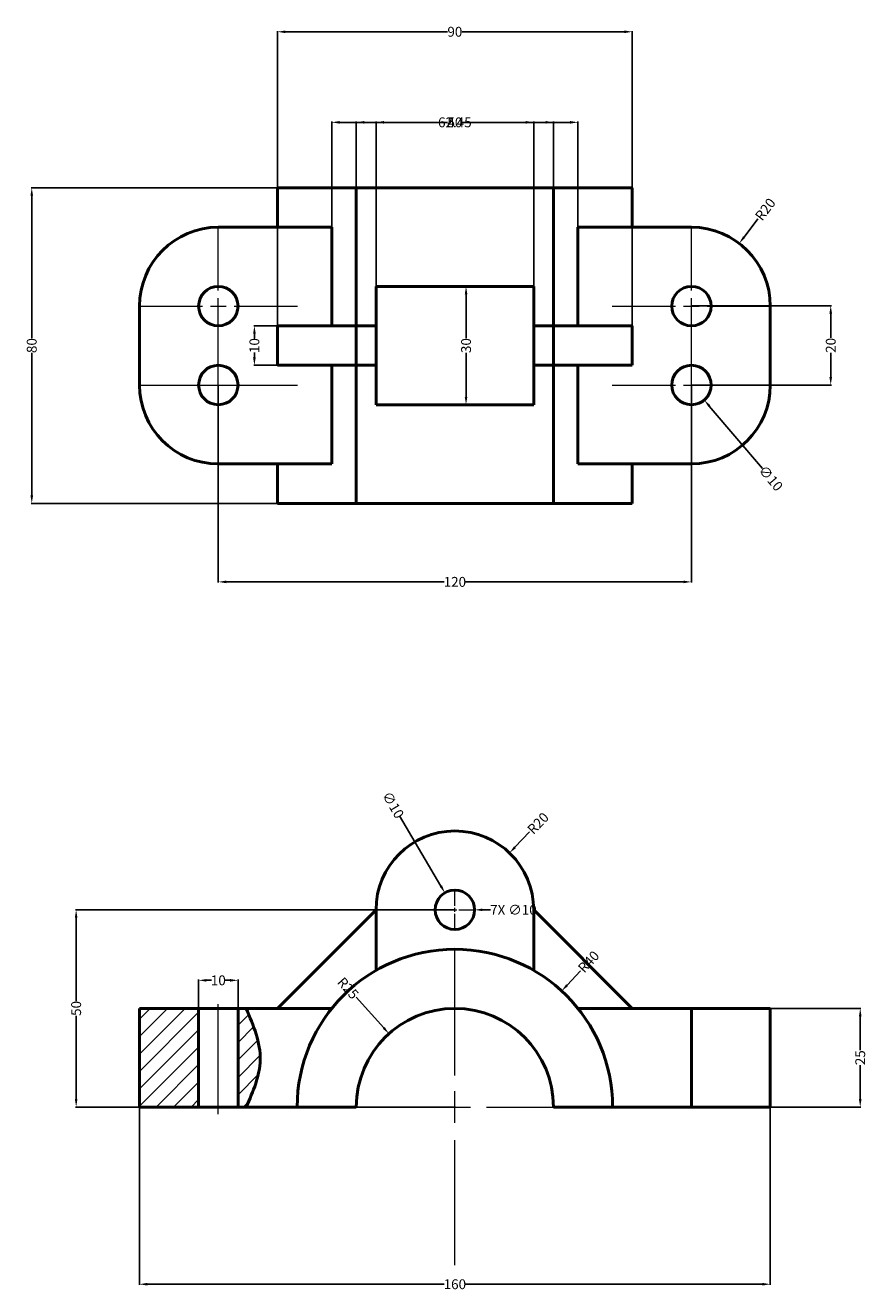
# Model space of a CAD drawing. Units: inches. Extents: x 156 to 369, y 156 to 477.
import ezdxf

# ---------------------------------------------------------------- set-up
doc = ezdxf.new("R2010")
doc.units = ezdxf.units.IN
doc.header["$MEASUREMENT"] = 0
doc.linetypes.add('CENTER', pattern=[50.8, 31.75, -6.35, 6.35, -6.35])
for name, color, linetype, lineweight in [('M-CNTR', 1, 'CENTER', 18), ('M-DIMS', 2, 'Continuous', 25), ('M-HATC', 8, 'Continuous', 18), ('M-OUTL', 7, 'Continuous', 50)]:
    doc.layers.add(name, color=color, linetype=linetype, lineweight=lineweight)
doc.styles.get("Standard").update_dxf_attribs({"font": 'arial.ttf'})
doc.dimstyles.get("Standard").update_dxf_attribs({"dimtxt": 2.5, "dimasz": 2, "dimexe": 0.18, "dimexo": 0.0625, "dimgap": 0.09, "dimtad": 0, "dimdec": 0, "dimzin": 0, "dimdsep": 46, "dimtxsty": 'Standard', "dimcen": 0.09, "dimadec": 0, "dimazin": 0, "dimtfac": 1, "dimtdec": 0, "dimtofl": 0, "dimtmove": 0, "dimatfit": 3, "dimfxl": 1, "dimtolj": 1, "dimtzin": 0, "dimarcsym": 0})

# ---------------------------------------------------------------- blocks, each defined once
blk = doc.blocks.new('*U1')
at = {"layer": 'M-CNTR', "color": 0, "transparency": 16777216}
blk.add_line((0, -14.29), (0, 13.61), dxfattribs=at)
blk = doc.blocks.new('*U2')
at = {"layer": 'M-CNTR', "color": 0, "transparency": 16777216}
for p, q in [((0, 1), (0, 5.12)), ((-5.12, 0), (-1, 0)), ((1, 0), (5.12, 0)), ((0, -5.12), (0, -1))]:
    blk.add_line(p, q, dxfattribs=at)
at = {"layer": 'M-CNTR', "color": 0, "linetype": 'Continuous', "transparency": 16777216}
for p, q in [((-0.5, 0), (0.5, 0)), ((0, -0.5), (0, 0.5))]:
    blk.add_line(p, q, dxfattribs=at)
blk = doc.blocks.new('*U3')
at = {"layer": 'M-CNTR', "color": 0, "transparency": 16777216}
for p, q in [((0, 4), (0, 20.12)), ((-20.12, 0), (-4, 0)), ((4, 0), (20.12, 0)), ((0, -20.12), (0, -4))]:
    blk.add_line(p, q, dxfattribs=at)
at = {"layer": 'M-CNTR', "color": 0, "linetype": 'Continuous', "transparency": 16777216}
for p, q in [((-2, 0), (2, 0)), ((0, -2), (0, 2))]:
    blk.add_line(p, q, dxfattribs=at)
blk = doc.blocks.new('*U4')
at = {"layer": 'M-CNTR', "color": 0, "transparency": 16777216}
for p, q in [((0, 4), (0, 20.12)), ((-20.12, 0), (-4, 0)), ((4, 0), (20.12, 0)), ((0, -20.12), (0, -4))]:
    blk.add_line(p, q, dxfattribs=at)
at = {"layer": 'M-CNTR', "color": 0, "linetype": 'Continuous', "transparency": 16777216}
for p, q in [((-2, 0), (2, 0)), ((0, -2), (0, 2))]:
    blk.add_line(p, q, dxfattribs=at)
blk = doc.blocks.new('*U5')
at = {"layer": 'M-CNTR', "color": 0, "transparency": 16777216}
for p, q in [((0, 4), (0, 20.12)), ((-20.12, 0), (-4, 0)), ((4, 0), (20.12, 0)), ((0, -20.12), (0, -4))]:
    blk.add_line(p, q, dxfattribs=at)
at = {"layer": 'M-CNTR', "color": 0, "linetype": 'Continuous', "transparency": 16777216}
for p, q in [((-2, 0), (2, 0)), ((0, -2), (0, 2))]:
    blk.add_line(p, q, dxfattribs=at)
blk = doc.blocks.new('*U6')
at = {"layer": 'M-CNTR', "color": 0, "transparency": 16777216}
for p, q in [((0, 4), (0, 20.12)), ((-20.12, 0), (-4, 0)), ((4, 0), (20.12, 0)), ((0, -20.12), (0, -4))]:
    blk.add_line(p, q, dxfattribs=at)
at = {"layer": 'M-CNTR', "color": 0, "linetype": 'Continuous', "transparency": 16777216}
for p, q in [((-2, 0), (2, 0)), ((0, -2), (0, 2))]:
    blk.add_line(p, q, dxfattribs=at)
blk = doc.blocks.new('*U7')
at = {"layer": 'M-CNTR', "color": 0, "transparency": 16777216}
for p, q in [((0, 1), (0, 5.12)), ((-5.12, 0), (-1, 0)), ((1, 0), (5.12, 0)), ((0, -5.12), (0, -1))]:
    blk.add_line(p, q, dxfattribs=at)
at = {"layer": 'M-CNTR', "color": 0, "linetype": 'Continuous', "transparency": 16777216}
for p, q in [((-0.5, 0), (0.5, 0)), ((0, -0.5), (0, 0.5))]:
    blk.add_line(p, q, dxfattribs=at)
blk = doc.blocks.new('*U8')
at = {"layer": 'M-CNTR', "color": 0, "transparency": 16777216}
for p, q in [((0, 8), (0, 40.12)), ((-40.12, 0), (-8, 0)), ((8, 0), (40.12, 0)), ((0, -40.12), (0, -8))]:
    blk.add_line(p, q, dxfattribs=at)
at = {"layer": 'M-CNTR', "color": 0, "linetype": 'Continuous', "transparency": 16777216}
for p, q in [((0, -4), (0, 4)), ((-4, 0), (4, 0))]:
    blk.add_line(p, q, dxfattribs=at)
blk = doc.blocks.new('*D9')
at = {"layer": 'Defpoints', "color": 0, "transparency": 16777216}
for p in [(184.76, 202.26), (344.76, 202.26), (344.76, 157.33)]:
    blk.add_point(p, dxfattribs=at)
at = {"layer": 'M-DIMS', "color": 0, "lineweight": -2, "transparency": 16777216}
for p, q in [((184.76, 202.19), (184.76, 157.15)), ((344.76, 202.19), (344.76, 157.15)), ((186.76, 157.33), (262.03, 157.33)), ((342.76, 157.33), (267.49, 157.33))]:
    blk.add_line(p, q, dxfattribs=at)
at = {"layer": 'M-DIMS', "color": 0, "transparency": 16777216}
for points in [[(186.76, 157.67), (186.76, 157), (184.76, 157.33)], [(342.76, 157.67), (342.76, 157), (344.76, 157.33)]]:
    blk.add_solid(points, dxfattribs=at)
at = {"layer": 'M-DIMS', "color": 0, "transparency": 16777216, "insert": (264.76, 157.33), "char_height": 2.5, "attachment_point": 5}
blk.add_mtext('\\A1;160', dxfattribs=at)
blk = doc.blocks.new('*D10')
at = {"layer": 'Defpoints', "color": 0, "transparency": 16777216}
for p in [(344.76, 227.26), (367.58, 227.26), (344.76, 202.26)]:
    blk.add_point(p, dxfattribs=at)
at = {"layer": 'M-DIMS', "color": 0, "lineweight": -2, "transparency": 16777216}
for p, q in [((344.83, 227.26), (367.76, 227.26)), ((367.58, 225.26), (367.58, 216.67)), ((367.58, 204.26), (367.58, 212.84)), ((344.83, 202.26), (367.76, 202.26))]:
    blk.add_line(p, q, dxfattribs=at)
at = {"layer": 'M-DIMS', "color": 0, "transparency": 16777216}
for points in [[(367.25, 225.26), (367.91, 225.26), (367.58, 227.26)], [(367.25, 204.26), (367.91, 204.26), (367.58, 202.26)]]:
    blk.add_solid(points, dxfattribs=at)
at = {"layer": 'M-DIMS', "color": 0, "transparency": 16777216, "insert": (367.58, 214.76), "char_height": 2.5, "attachment_point": 5, "rotation": 90}
blk.add_mtext('\\A1;25', dxfattribs=at)
blk = doc.blocks.new('*D11')
at = {"layer": 'Defpoints', "color": 0, "transparency": 16777216}
for p in [(264.76, 252.26), (168.7, 202.26), (264.76, 202.26)]:
    blk.add_point(p, dxfattribs=at)
at = {"layer": 'M-DIMS', "color": 0, "lineweight": -2, "transparency": 16777216}
for p, q in [((264.7, 252.26), (168.52, 252.26)), ((168.7, 250.26), (168.7, 229.13)), ((168.7, 204.26), (168.7, 225.38)), ((264.7, 202.26), (168.52, 202.26))]:
    blk.add_line(p, q, dxfattribs=at)
at = {"layer": 'M-DIMS', "color": 0, "transparency": 16777216}
for points in [[(168.37, 250.26), (169.03, 250.26), (168.7, 252.26)], [(168.37, 204.26), (169.03, 204.26), (168.7, 202.26)]]:
    blk.add_solid(points, dxfattribs=at)
at = {"layer": 'M-DIMS', "color": 0, "transparency": 16777216, "insert": (168.7, 227.26), "char_height": 2.5, "attachment_point": 5, "rotation": 90}
blk.add_mtext('\\A1;50', dxfattribs=at)
blk = doc.blocks.new('*D12')
at = {"layer": 'Defpoints', "color": 0, "transparency": 16777216}
for p in [(209.76, 234.38), (199.76, 227.26), (209.76, 227.26)]:
    blk.add_point(p, dxfattribs=at)
at = {"layer": 'M-DIMS', "color": 0, "lineweight": -2, "transparency": 16777216}
for p, q in [((199.76, 227.32), (199.76, 234.56)), ((201.76, 234.38), (203, 234.38)), ((207.76, 234.38), (206.52, 234.38)), ((209.76, 227.32), (209.76, 234.56))]:
    blk.add_line(p, q, dxfattribs=at)
at = {"layer": 'M-DIMS', "color": 0, "transparency": 16777216}
for points in [[(201.76, 234.71), (201.76, 234.04), (199.76, 234.38)], [(207.76, 234.71), (207.76, 234.04), (209.76, 234.38)]]:
    blk.add_solid(points, dxfattribs=at)
at = {"layer": 'M-DIMS', "color": 0, "transparency": 16777216, "insert": (204.76, 234.38), "char_height": 2.5, "attachment_point": 5}
blk.add_mtext('\\A1;10', dxfattribs=at)
blk = doc.blocks.new('*D13')
at = {"layer": 'Defpoints', "color": 0, "transparency": 16777216}
for p in [(278.62, 266.68), (264.76, 252.26)]:
    blk.add_point(p, dxfattribs=at)
at = {"layer": 'M-DIMS', "color": 0, "lineweight": -2, "transparency": 16777216}
for p, q in [((283.73, 271.99), (280.01, 268.12)), ((264.67, 252.26), (264.85, 252.26)), ((264.76, 252.17), (264.76, 252.35))]:
    blk.add_line(p, q, dxfattribs=at)
at = {"layer": 'M-DIMS', "color": 0, "transparency": 16777216}
blk.add_solid([(279.77, 268.35), (280.25, 267.89), (278.62, 266.68)], dxfattribs=at)
at = {"layer": 'M-DIMS', "color": 0, "transparency": 16777216, "insert": (285.86, 274.2), "char_height": 2.5, "attachment_point": 5, "rotation": 46.136}
blk.add_mtext('\\A1;R20', dxfattribs=at)
blk = doc.blocks.new('*D14')
at = {"layer": 'Defpoints', "color": 0, "transparency": 16777216}
for p in [(291.86, 231.68), (264.76, 202.26)]:
    blk.add_point(p, dxfattribs=at)
at = {"layer": 'M-DIMS', "color": 0, "lineweight": -2, "transparency": 16777216}
for p, q in [((296.61, 236.83), (293.22, 233.15)), ((264.67, 202.26), (264.85, 202.26)), ((264.76, 202.17), (264.76, 202.35))]:
    blk.add_line(p, q, dxfattribs=at)
at = {"layer": 'M-DIMS', "color": 0, "transparency": 16777216}
blk.add_solid([(292.97, 233.37), (293.46, 232.92), (291.86, 231.68)], dxfattribs=at)
at = {"layer": 'M-DIMS', "color": 0, "transparency": 16777216, "insert": (298.69, 239.09), "char_height": 2.5, "attachment_point": 5, "rotation": 47.3487}
blk.add_mtext('\\A1;R40', dxfattribs=at)
blk = doc.blocks.new('*D15')
at = {"layer": 'Defpoints', "color": 0, "transparency": 16777216}
for p in [(248.05, 220.84), (264.76, 202.26)]:
    blk.add_point(p, dxfattribs=at)
at = {"layer": 'M-DIMS', "color": 0, "lineweight": -2, "transparency": 16777216}
for p, q in [((239.72, 230.1), (246.71, 222.33)), ((264.67, 202.26), (264.85, 202.26)), ((264.76, 202.17), (264.76, 202.35))]:
    blk.add_line(p, q, dxfattribs=at)
at = {"layer": 'M-DIMS', "color": 0, "transparency": 16777216}
blk.add_solid([(246.96, 222.55), (246.46, 222.11), (248.05, 220.84)], dxfattribs=at)
at = {"layer": 'M-DIMS', "color": 0, "transparency": 16777216, "insert": (237.66, 232.4), "char_height": 2.5, "attachment_point": 5, "rotation": 311.9649}
blk.add_mtext('\\A1;R25', dxfattribs=at)
blk = doc.blocks.new('*D16')
at = {"layer": 'Defpoints', "color": 0, "transparency": 16777216}
for p in [(262.23, 256.56), (267.3, 247.95)]:
    blk.add_point(p, dxfattribs=at)
at = {"layer": 'M-DIMS', "color": 0, "lineweight": -2, "transparency": 16777216}
for p, q in [((250.75, 276.06), (261.21, 258.29)), ((264.67, 252.26), (264.85, 252.26)), ((264.76, 252.17), (264.76, 252.35))]:
    blk.add_line(p, q, dxfattribs=at)
at = {"layer": 'M-DIMS', "color": 0, "transparency": 16777216}
blk.add_solid([(261.5, 258.46), (260.92, 258.12), (262.23, 256.56)], dxfattribs=at)
at = {"layer": 'M-DIMS', "color": 0, "transparency": 16777216, "insert": (249.11, 278.85), "char_height": 2.5, "attachment_point": 5, "rotation": 300.4828}
blk.add_mtext('\\A1;∅10', dxfattribs=at)
blk = doc.blocks.new('*D17')
at = {"layer": 'Defpoints', "color": 0, "transparency": 16777216}
for p in [(204.76, 385.31), (324.76, 385.31), (324.76, 335.4)]:
    blk.add_point(p, dxfattribs=at)
at = {"layer": 'M-DIMS', "color": 0, "lineweight": -2, "transparency": 16777216}
for p, q in [((204.76, 385.25), (204.76, 335.22)), ((324.76, 385.25), (324.76, 335.22)), ((206.76, 335.4), (262.03, 335.4)), ((322.76, 335.4), (267.49, 335.4))]:
    blk.add_line(p, q, dxfattribs=at)
at = {"layer": 'M-DIMS', "color": 0, "transparency": 16777216}
for points in [[(206.76, 335.73), (206.76, 335.06), (204.76, 335.4)], [(322.76, 335.73), (322.76, 335.06), (324.76, 335.4)]]:
    blk.add_solid(points, dxfattribs=at)
at = {"layer": 'M-DIMS', "color": 0, "transparency": 16777216, "insert": (264.76, 335.4), "char_height": 2.5, "attachment_point": 5}
blk.add_mtext('\\A1;120', dxfattribs=at)
blk = doc.blocks.new('*D18')
at = {"layer": 'Defpoints', "color": 0, "transparency": 16777216}
for p in [(324.76, 405.43), (324.76, 385.31), (360.1, 385.31)]:
    blk.add_point(p, dxfattribs=at)
at = {"layer": 'M-DIMS', "color": 0, "lineweight": -2, "transparency": 16777216}
for p, q in [((324.83, 405.43), (360.28, 405.43)), ((360.1, 403.43), (360.1, 397.27)), ((360.1, 387.31), (360.1, 393.48)), ((324.83, 385.31), (360.28, 385.31))]:
    blk.add_line(p, q, dxfattribs=at)
at = {"layer": 'M-DIMS', "color": 0, "transparency": 16777216}
for points in [[(359.76, 403.43), (360.43, 403.43), (360.1, 405.43)], [(359.76, 387.31), (360.43, 387.31), (360.1, 385.31)]]:
    blk.add_solid(points, dxfattribs=at)
at = {"layer": 'M-DIMS', "color": 0, "transparency": 16777216, "insert": (360.1, 395.37), "char_height": 2.5, "attachment_point": 5, "rotation": 90}
blk.add_mtext('\\A1;20', dxfattribs=at)
blk = doc.blocks.new('*D19')
at = {"layer": 'Defpoints', "color": 0, "transparency": 16777216}
for p in [(309.76, 474.87), (219.76, 395.31), (309.76, 395.31)]:
    blk.add_point(p, dxfattribs=at)
at = {"layer": 'M-DIMS', "color": 0, "lineweight": -2, "transparency": 16777216}
for p, q in [((219.76, 395.38), (219.76, 475.05)), ((221.76, 474.87), (262.89, 474.87)), ((307.76, 474.87), (266.64, 474.87)), ((309.76, 395.38), (309.76, 475.05))]:
    blk.add_line(p, q, dxfattribs=at)
at = {"layer": 'M-DIMS', "color": 0, "transparency": 16777216}
for points in [[(221.76, 475.2), (221.76, 474.54), (219.76, 474.87)], [(307.76, 475.2), (307.76, 474.54), (309.76, 474.87)]]:
    blk.add_solid(points, dxfattribs=at)
at = {"layer": 'M-DIMS', "color": 0, "transparency": 16777216, "insert": (264.76, 474.87), "char_height": 2.5, "attachment_point": 5}
blk.add_mtext('\\A1;90', dxfattribs=at)
blk = doc.blocks.new('*D20')
at = {"layer": 'Defpoints', "color": 0, "transparency": 16777216}
for p in [(219.76, 435.31), (157.44, 355.31), (219.76, 355.31)]:
    blk.add_point(p, dxfattribs=at)
at = {"layer": 'M-DIMS', "color": 0, "lineweight": -2, "transparency": 16777216}
for p, q in [((219.7, 435.31), (157.26, 435.31)), ((157.44, 433.31), (157.44, 397.19)), ((157.44, 357.31), (157.44, 393.44)), ((219.7, 355.31), (157.26, 355.31))]:
    blk.add_line(p, q, dxfattribs=at)
at = {"layer": 'M-DIMS', "color": 0, "transparency": 16777216}
for points in [[(157.11, 433.31), (157.78, 433.31), (157.44, 435.31)], [(157.11, 357.31), (157.78, 357.31), (157.44, 355.31)]]:
    blk.add_solid(points, dxfattribs=at)
at = {"layer": 'M-DIMS', "color": 0, "transparency": 16777216, "insert": (157.44, 395.31), "char_height": 2.5, "attachment_point": 5, "rotation": 90}
blk.add_mtext('\\A1;80', dxfattribs=at)
blk = doc.blocks.new('*D21')
at = {"layer": 'Defpoints', "color": 0, "transparency": 16777216}
for p in [(284.76, 410.31), (267.6, 380.31), (284.76, 380.31)]:
    blk.add_point(p, dxfattribs=at)
at = {"layer": 'M-DIMS', "color": 0, "lineweight": -2, "transparency": 16777216}
for p, q in [((284.7, 410.31), (267.42, 410.31)), ((267.6, 408.31), (267.6, 397.19)), ((267.6, 382.31), (267.6, 393.44)), ((284.7, 380.31), (267.42, 380.31))]:
    blk.add_line(p, q, dxfattribs=at)
at = {"layer": 'M-DIMS', "color": 0, "transparency": 16777216}
for points in [[(267.27, 408.31), (267.93, 408.31), (267.6, 410.31)], [(267.27, 382.31), (267.93, 382.31), (267.6, 380.31)]]:
    blk.add_solid(points, dxfattribs=at)
at = {"layer": 'M-DIMS', "color": 0, "transparency": 16777216, "insert": (267.6, 395.31), "char_height": 2.5, "attachment_point": 5, "rotation": 90}
blk.add_mtext('\\A1;30', dxfattribs=at)
blk = doc.blocks.new('*D22')
at = {"layer": 'Defpoints', "color": 0, "transparency": 16777216}
for p in [(219.76, 400.31), (213.91, 390.31), (219.76, 390.31)]:
    blk.add_point(p, dxfattribs=at)
at = {"layer": 'M-DIMS', "color": 0, "lineweight": -2, "transparency": 16777216}
for p, q in [((219.7, 400.31), (213.73, 400.31)), ((213.91, 398.31), (213.91, 397.07)), ((213.91, 392.31), (213.91, 393.55)), ((219.7, 390.31), (213.73, 390.31))]:
    blk.add_line(p, q, dxfattribs=at)
at = {"layer": 'M-DIMS', "color": 0, "transparency": 16777216}
for points in [[(213.58, 398.31), (214.25, 398.31), (213.91, 400.31)], [(213.58, 392.31), (214.25, 392.31), (213.91, 390.31)]]:
    blk.add_solid(points, dxfattribs=at)
at = {"layer": 'M-DIMS', "color": 0, "transparency": 16777216, "insert": (213.91, 395.31), "char_height": 2.5, "attachment_point": 5, "rotation": 90}
blk.add_mtext('\\A1;10', dxfattribs=at)
blk = doc.blocks.new('*D23')
at = {"layer": 'Defpoints', "color": 0, "transparency": 16777216}
for p in [(336.9, 421.21), (324.76, 405.31)]:
    blk.add_point(p, dxfattribs=at)
at = {"layer": 'M-DIMS', "color": 0, "lineweight": -2, "transparency": 16777216}
for p, q in [((341.63, 427.42), (338.11, 422.8)), ((324.67, 405.31), (324.85, 405.31)), ((324.76, 405.22), (324.76, 405.4))]:
    blk.add_line(p, q, dxfattribs=at)
at = {"layer": 'M-DIMS', "color": 0, "transparency": 16777216}
blk.add_solid([(337.84, 423.01), (338.37, 422.6), (336.9, 421.21)], dxfattribs=at)
at = {"layer": 'M-DIMS', "color": 0, "transparency": 16777216, "insert": (343.5, 429.87), "char_height": 2.5, "attachment_point": 5, "rotation": 52.6551}
blk.add_mtext('\\A1;R20', dxfattribs=at)
blk = doc.blocks.new('*D24')
at = {"layer": 'Defpoints', "color": 0, "transparency": 16777216}
for p in [(321.52, 389.12), (328.01, 381.51)]:
    blk.add_point(p, dxfattribs=at)
at = {"layer": 'M-DIMS', "color": 0, "lineweight": -2, "transparency": 16777216}
for p, q in [((324.67, 385.31), (324.85, 385.31)), ((324.76, 385.22), (324.76, 385.4)), ((342.8, 364.14), (329.3, 379.99))]:
    blk.add_line(p, q, dxfattribs=at)
at = {"layer": 'M-DIMS', "color": 0, "transparency": 16777216}
blk.add_solid([(329.56, 380.2), (329.05, 379.77), (328.01, 381.51)], dxfattribs=at)
at = {"layer": 'M-DIMS', "color": 0, "transparency": 16777216, "insert": (344.9, 361.68), "char_height": 2.5, "attachment_point": 5, "rotation": 310.4308}
blk.add_mtext('\\A1;∅10', dxfattribs=at)
blk = doc.blocks.new('*D25')
at = {"layer": 'Defpoints', "color": 0, "transparency": 16777216}
for p in [(284.76, 451.91), (244.76, 410.31), (284.76, 410.31)]:
    blk.add_point(p, dxfattribs=at)
at = {"layer": 'M-DIMS', "color": 0, "lineweight": -2, "transparency": 16777216}
for p, q in [((244.76, 410.38), (244.76, 452.09)), ((246.76, 451.91), (262.84, 451.91)), ((282.76, 451.91), (266.69, 451.91)), ((284.76, 410.38), (284.76, 452.09))]:
    blk.add_line(p, q, dxfattribs=at)
at = {"layer": 'M-DIMS', "color": 0, "transparency": 16777216}
for points in [[(246.76, 452.25), (246.76, 451.58), (244.76, 451.91)], [(282.76, 452.25), (282.76, 451.58), (284.76, 451.91)]]:
    blk.add_solid(points, dxfattribs=at)
at = {"layer": 'M-DIMS', "color": 0, "transparency": 16777216, "insert": (264.76, 451.91), "char_height": 2.5, "attachment_point": 5}
blk.add_mtext('\\A1;40', dxfattribs=at)
blk = doc.blocks.new('*D26')
at = {"layer": 'Defpoints', "color": 0, "transparency": 16777216}
for p in [(289.76, 451.91), (239.76, 435.31), (289.76, 435.31)]:
    blk.add_point(p, dxfattribs=at)
at = {"layer": 'M-DIMS', "color": 0, "lineweight": -2, "transparency": 16777216}
for p, q in [((239.76, 435.38), (239.76, 452.09)), ((241.76, 451.91), (262.89, 451.91)), ((287.76, 451.91), (266.64, 451.91)), ((289.76, 435.38), (289.76, 452.09))]:
    blk.add_line(p, q, dxfattribs=at)
at = {"layer": 'M-DIMS', "color": 0, "transparency": 16777216}
for points in [[(241.76, 452.25), (241.76, 451.58), (239.76, 451.91)], [(287.76, 452.25), (287.76, 451.58), (289.76, 451.91)]]:
    blk.add_solid(points, dxfattribs=at)
at = {"layer": 'M-DIMS', "color": 0, "transparency": 16777216, "insert": (264.76, 451.91), "char_height": 2.5, "attachment_point": 5}
blk.add_mtext('\\A1;50', dxfattribs=at)
blk = doc.blocks.new('*D27')
at = {"layer": 'Defpoints', "color": 0, "transparency": 16777216}
for p in [(295.99, 451.91), (233.54, 425.31), (295.99, 425.31)]:
    blk.add_point(p, dxfattribs=at)
at = {"layer": 'M-DIMS', "color": 0, "lineweight": -2, "transparency": 16777216}
for p, q in [((233.54, 425.38), (233.54, 452.09)), ((235.54, 451.91), (260.44, 451.91)), ((293.99, 451.91), (269.09, 451.91)), ((295.99, 425.38), (295.99, 452.09))]:
    blk.add_line(p, q, dxfattribs=at)
at = {"layer": 'M-DIMS', "color": 0, "transparency": 16777216}
for points in [[(235.54, 452.25), (235.54, 451.58), (233.54, 451.91)], [(293.99, 452.25), (293.99, 451.58), (295.99, 451.91)]]:
    blk.add_solid(points, dxfattribs=at)
at = {"layer": 'M-DIMS', "color": 0, "transparency": 16777216, "insert": (264.76, 451.91), "char_height": 2.5, "attachment_point": 5}
blk.add_mtext('\\A1;62.45', dxfattribs=at)
blk = doc.blocks.new('*D28')
at = {"layer": 'Defpoints', "color": 0, "transparency": 16777216}
for p in [(259.76, 252.26), (269.76, 252.25)]:
    blk.add_point(p, dxfattribs=at)
at = {"layer": 'M-DIMS', "color": 0, "lineweight": -2, "transparency": 16777216}
for p, q in [((264.67, 252.26), (264.85, 252.26)), ((264.76, 252.17), (264.76, 252.35)), ((273.76, 252.25), (271.76, 252.25))]:
    blk.add_line(p, q, dxfattribs=at)
at = {"layer": 'M-DIMS', "color": 0, "transparency": 16777216}
blk.add_solid([(271.76, 252.59), (271.76, 251.92), (269.76, 252.25)], dxfattribs=at)
at = {"layer": 'M-DIMS', "color": 0, "transparency": 16777216, "insert": (279.61, 252.25), "char_height": 2.5, "attachment_point": 5, "rotation": 359.9947}
blk.add_mtext('\\A1;7X ∅10', dxfattribs=at)

msp = doc.modelspace()

# ---------------------------------------------------------------- hatches: boundary and pattern name
at = {"layer": 'M-HATC'}
h = msp.add_hatch(dxfattribs=at)
h.set_pattern_fill('ANSI31', color=256, scale=25)
edge = h.paths.add_edge_path()
edge.add_spline(control_points=[(211.829, 202.255), (213.575, 206.24), (217.21, 214.532), (213.669, 222.905), (211.829, 227.255)], knot_values=[0, 0, 0, 0, 12.4957208, 26.0084045, 26.0084045, 26.0084045, 26.0084045], degree=3, periodic=0)
edge.add_line((211.829, 227.255), (209.763, 227.255))
edge.add_line((209.763, 227.255), (209.763, 202.255))
edge.add_line((209.763, 202.255), (211.829, 202.255))
h.paths.add_polyline_path([(199.763, 227.255), (194.763, 227.255), (184.763, 227.255), (184.763, 202.255), (199.763, 202.255)])

# ---------------------------------------------------------------- linework, layer by layer
at = {"layer": 'M-OUTL'}
for p, q in [((219.763, 435.314), (309.763, 435.314)), ((219.763, 425.314), (219.763, 435.314)), ((219.763, 425.314), (219.763, 435.314)), ((239.763, 435.314), (239.763, 355.314)), ((289.763, 435.314), (289.763, 355.314)), ((309.763, 425.314), (309.763, 435.314)), ((309.763, 425.314), (309.763, 435.314)), ((233.538, 425.314), (204.763, 425.314)), ((233.538, 425.314), (233.538, 400.314)), ((233.538, 400.314), (233.538, 425.314)), ((233.538, 400.314), (233.538, 425.314)), ((295.988, 400.314), (295.988, 425.314)), ((295.988, 425.314), (324.763, 425.314)), ((284.763, 410.314), (244.763, 410.314)), ((244.763, 380.314), (244.763, 410.314)), ((284.763, 380.314), (284.763, 410.314)), ((184.763, 385.314), (184.763, 405.314)), ((344.763, 385.314), (344.763, 405.314)), ((244.763, 400.314), (219.763, 400.314)), ((219.763, 390.314), (219.763, 400.314)), ((219.763, 390.314), (219.763, 400.314)), ((309.763, 400.314), (284.763, 400.314)), ((284.763, 400.314), (309.763, 400.314)), ((309.763, 390.314), (309.763, 400.314)), ((219.763, 395.314), (219.763, 390.314)), ((309.763, 395.314), (309.763, 390.314)), ((244.763, 390.314), (219.763, 390.314)), ((233.538, 365.314), (233.538, 390.314)), ((233.538, 365.314), (233.538, 390.314)), ((309.763, 390.314), (284.763, 390.314)), ((284.763, 390.314), (309.763, 390.314)), ((295.988, 365.314), (295.988, 390.314)), ((244.763, 380.314), (284.763, 380.314)), ((219.763, 365.314), (204.763, 365.314)), ((219.763, 355.314), (219.763, 365.314)), ((219.763, 355.314), (219.763, 365.314)), ((219.763, 365.314), (233.538, 365.314)), ((309.763, 365.314), (295.988, 365.314)), ((309.763, 355.314), (309.763, 365.314)), ((309.763, 355.314), (309.763, 365.314)), ((309.763, 365.314), (324.763, 365.314)), ((264.763, 355.314), (219.763, 355.314)), ((219.763, 355.314), (269.141, 355.314)), ((309.763, 355.314), (260.385, 355.314)), ((309.763, 355.314), (264.763, 355.314)), ((264.763, 355.314), (309.763, 355.314)), ((244.763, 252.255), (219.763, 227.255)), ((244.763, 252.255), (244.763, 236.896)), ((244.763, 252.255), (244.763, 236.896)), ((269.763, 252.255), (269.762, 252.316)), ((284.763, 252.255), (309.763, 227.255)), ((284.763, 252.255), (284.763, 236.896)), ((284.763, 252.255), (284.763, 236.896)), ((184.763, 202.255), (184.763, 227.255)), ((184.763, 227.255), (194.763, 227.255)), ((199.763, 202.255), (199.763, 227.255)), ((209.763, 202.255), (209.763, 227.255)), ((324.763, 202.255), (324.763, 227.255)), ((344.763, 227.255), (334.763, 227.255)), ((344.763, 202.255), (344.763, 227.255)), ((204.763, 202.255), (184.763, 202.255)), ((211.829, 202.255), (204.763, 202.255))]:
    msp.add_line(p, q, dxfattribs=at)
for points in [[(194.763, 227.255), (233.538, 227.255)], [(295.988, 227.255), (334.763, 227.255)], [(239.763, 202.255), (194.763, 202.255)], [(324.763, 202.255), (289.763, 202.255)], [(344.763, 202.255), (324.763, 202.255)]]:
    msp.add_lwpolyline(points, dxfattribs=at)
for centre in [(204.763, 405.314), (324.763, 405.314), (324.763, 405.314), (204.763, 385.314), (324.763, 385.314), (324.763, 385.314), (264.763, 252.255)]:
    msp.add_circle(centre, 5, dxfattribs=at)
for centre, radius, start, end in [((204.763, 405.314), 20, 90, 180), ((324.763, 405.314), 20, 360, 90), ((204.763, 385.314), 20, 180, 270), ((324.763, 385.314), 20, 270, 360), ((264.763, 252.255), 20, 0, 180), ((264.763, 202.255), 40, 0, 180), ((264.763, 202.255), 25, 0, 180)]:
    msp.add_arc(centre, radius, start, end, dxfattribs=at)
msp.add_open_spline([(211.829, 227.255), (213.669, 222.905), (217.21, 214.532), (213.575, 206.24), (211.829, 202.255)], degree=3, knots=[0, 0, 0, 0, 13.5126838, 26.0084045, 26.0084045, 26.0084045, 26.0084045], dxfattribs=at)

# ---------------------------------------------------------------- block references
at = {"layer": 'M-CNTR'}
for name, p in [('*U4', (204.763, 405.314)), ('*U5', (324.763, 405.314)), ('*U3', (204.763, 385.314)), ('*U6', (324.763, 385.314)), ('*U2', (204.763, 385.314)), ('*U7', (264.763, 252.255)), ('*U8', (264.763, 202.255)), ('*U1', (204.763, 214.755))]:
    msp.add_blockref(name, p, dxfattribs=at)

# ---------------------------------------------------------------- dimensions: what is measured, and where the dimension line sits
at = {"layer": 'M-DIMS'}
for base, p1, p2, override, picture, middle in [((309.763, 474.871), (219.763, 395.314), (309.763, 395.314), {"dimclrd": 0, "dimclre": 0, "dimclrt": 0}, '*D19', (264.763, 474.871)), ((295.988, 451.914), (233.538, 425.314), (295.988, 425.314), {"dimdec": 2, "dimlfac": 1, "dimrnd": 0, "dimzin": 0, "dimdsep": 46, "dimlunit": 2}, '*D27', (264.763, 451.914)), ((289.763, 451.914), (239.763, 435.314), (289.763, 435.314), {"dimdec": 0, "dimlfac": 1, "dimrnd": 0, "dimzin": 0, "dimdsep": 46, "dimlunit": 2}, '*D26', (264.763, 451.914)), ((284.763, 451.914), (244.763, 410.314), (284.763, 410.314), {"dimdec": 0, "dimlfac": 1, "dimrnd": 0, "dimzin": 0, "dimdsep": 46, "dimlunit": 2}, '*D25', (264.763, 451.914)), ((324.763, 335.396), (204.763, 385.314), (324.763, 385.314), {"dimclrd": 0, "dimclre": 0, "dimclrt": 0}, '*D17', (264.763, 335.396)), ((209.763, 234.376), (199.763, 227.255), (209.763, 227.255), {"dimclrd": 0, "dimclre": 0, "dimclrt": 0}, '*D12', (204.763, 234.376)), ((344.763, 157.333), (184.763, 202.255), (344.763, 202.255), {"dimclrd": 0, "dimclre": 0, "dimclrt": 0}, '*D9', (264.763, 157.333))]:
    dim = msp.add_linear_dim(base=base, p1=p1, p2=p2, dimstyle='Standard', override=override, dxfattribs=at)
    dim.commit()
    dim.dimension.update_dxf_attribs({"geometry": picture, "text_midpoint": middle})
for base, p1, p2, picture, middle in [((157.443, 355.314), (219.763, 435.314), (219.763, 355.314), '*D20', (157.443, 395.314)), ((267.599, 380.314), (284.763, 410.314), (284.763, 380.314), '*D21', (267.599, 395.314)), ((360.097, 385.314), (324.763, 405.434), (324.763, 385.314), '*D18', (360.097, 395.374)), ((213.915, 390.314), (219.763, 400.314), (219.763, 390.314), '*D22', (213.915, 395.314)), ((168.699, 202.255), (264.763, 252.255), (264.763, 202.255), '*D11', (168.699, 227.255)), ((367.581, 227.255), (344.763, 202.255), (344.763, 227.255), '*D10', (367.581, 214.755))]:
    dim = msp.add_linear_dim(base=base, p1=p1, p2=p2, angle=90, dimstyle='Standard', override={"dimclrd": 0, "dimclre": 0, "dimclrt": 0}, dxfattribs=at)
    dim.commit()
    dim.dimension.update_dxf_attribs({"geometry": picture, "text_midpoint": middle})
for center, mpoint, picture, middle in [((324.763, 405.314), (336.895, 421.214), '*D23', (343.498, 429.867)), ((264.763, 252.255), (278.622, 266.675), '*D13', (285.858, 274.204)), ((264.763, 202.255), (291.864, 231.675), '*D14', (298.694, 239.089)), ((264.763, 202.255), (248.046, 220.844), '*D15', (237.658, 232.395))]:
    dim = msp.add_radius_dim(center=center, mpoint=mpoint, dimstyle='Standard', override={"dimclrd": 0, "dimclre": 0, "dimclrt": 0}, dxfattribs=at)
    dim.commit()
    dim.dimension.update_dxf_attribs({"geometry": picture, "text_midpoint": middle, "dimtype": 164})
for p1, p2, picture, middle in [((321.52, 389.12), (328.005, 381.508), '*D24', (344.9, 361.678)), ((267.299, 247.947), (262.226, 256.564), '*D16', (249.109, 278.848))]:
    dim = msp.add_diameter_dim_2p(p1=p1, p2=p2, dimstyle='Standard', override={"dimclrd": 0, "dimclre": 0, "dimclrt": 0}, dxfattribs=at)
    dim.commit()
    dim.dimension.update_dxf_attribs({"geometry": picture, "text_midpoint": middle, "dimtype": 163})
dim = msp.add_diameter_dim_2p(p1=(259.763, 252.256), p2=(269.763, 252.255), text='7X <>', dimstyle='Standard', override={"dimdec": 0, "dimlfac": 1, "dimrnd": 0, "dimzin": 0, "dimdsep": 46, "dimlunit": 2}, dxfattribs=at)
dim.commit()
dim.dimension.update_dxf_attribs({"geometry": '*D28', "text_midpoint": (279.608, 252.254)})

doc.saveas('drawing.dxf')
